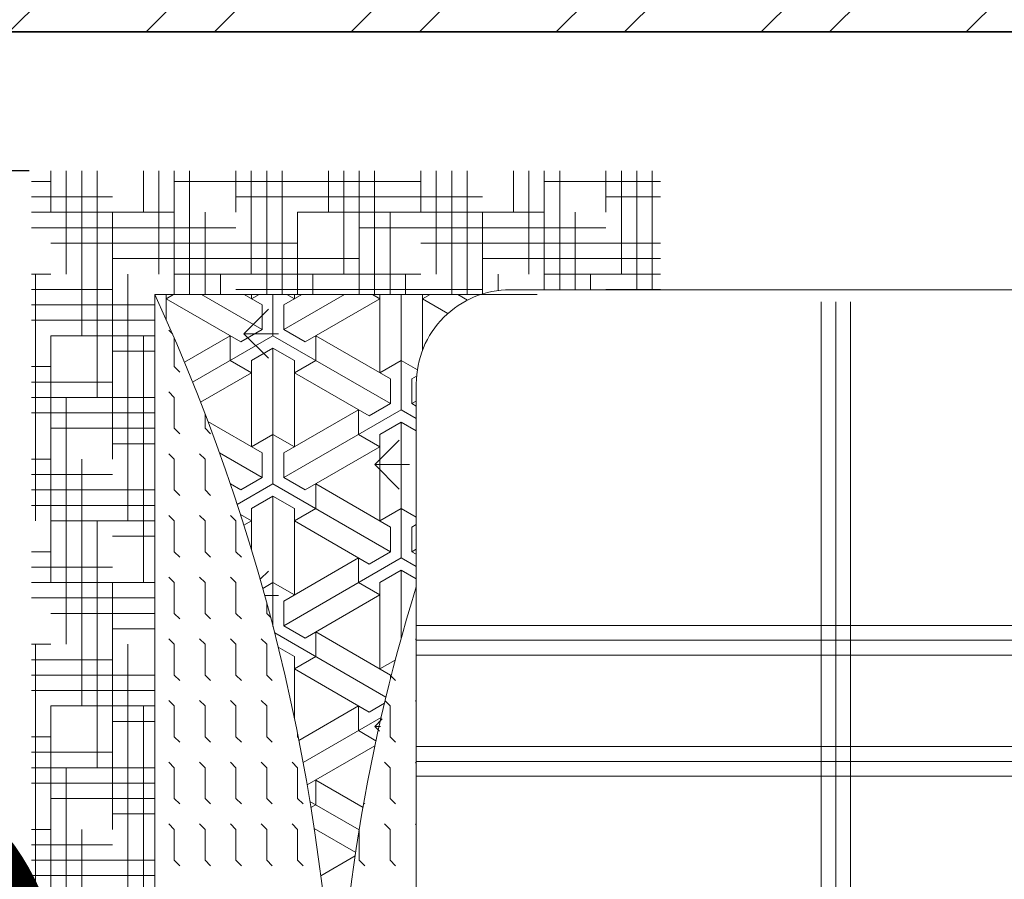
# Model space of a CAD drawing. Units: inches. Extents: x -90 to 536, y -553 to 299.
# Tile 7 of 27: x 96 to 122, y -362 to -339. Entities that reach past the tile are written whole.
import ezdxf

# ---------------------------------------------------------------- set-up
doc = ezdxf.new("R2010")
doc.units = ezdxf.units.IN
for name, color, linetype, lineweight in [('A-ANNO-DIMS', 2, 'Continuous', 18), ('A-WALL-PATT', 252, 'Continuous', 13), ('Furniture', 2, 'Continuous', 18), ('Inner Wall', 5, 'Continuous', 35)]:
    doc.layers.add(name, color=color, linetype=linetype, lineweight=lineweight)
doc.styles.get("Standard").update_dxf_attribs({"font": 'arial.ttf'})
doc.dimstyles.get("Standard").update_dxf_attribs({"dimtxt": 18, "dimasz": 12, "dimexe": 0.18, "dimexo": 0.0625, "dimgap": 0.09, "dimtad": 0, "dimtih": 1, "dimtoh": 1, "dimdec": 0, "dimzin": 0, "dimdsep": 46, "dimlunit": 3, "dimtxsty": 'Standard', "dimcen": 0.09, "dimadec": 0, "dimazin": 0, "dimtfac": 1, "dimtdec": 0, "dimtofl": 0, "dimtmove": 0, "dimatfit": 3, "dimfxl": 1, "dimtolj": 1, "dimtzin": 0, "dimarcsym": 0})

# ---------------------------------------------------------------- blocks, each defined once
blk = doc.blocks.new('A$C62731D1C')
for p, q in [((0.09627, 0.38824, 0.68571), (0.09627, 2.14084, 0.68571)), ((0.46643, 1.44371, 0.68571), (0.46643, 0.31204, 0.68571)), ((0.47843, 1.44371, 0.68571), (0.47843, 0.31204, 0.68571)), ((0.49043, 1.44371, 0.68571), (0.49043, 0.31204, 0.68571)), ((0.36826, 1.4076, 0.68571), (0.36826, 0.31204, 0.68571)), ((0.38026, 1.4076, 0.68571), (0.38026, 0.31204, 0.68571)), ((0.39226, 1.4076, 0.68571), (0.39226, 0.31204, 0.68571)), ((0.10613, 0.66415, 0.68571), (1.46095, 0.66415, 0.68571)), ((0.10613, 0.65215, 0.68571), (1.46095, 0.65215, 0.68571)), ((0.10613, 0.64015, 0.68571), (1.46095, 0.64015, 0.68571)), ((0, 0.50327, 0.68571), (0.09627, 0.50327, 0.68571)), ((0.0085, 0.41577, 0.68571), (0.0085, 0.50998, 0.68571)), ((0.021, 0.46577, 0.68571), (0.021, 0.50998, 0.68571)), ((0.0585, 0.31577, 0.68571), (0.0585, 0.50998, 0.68571)), ((0.071, 0.36577, 0.68571), (0.071, 0.50998, 0.68571)), ((0.0835, 0.41577, 0.68571), (0.0835, 0.50998, 0.68571)), ((0.096, 0.46577, 0.68571), (0.096, 0.50998, 0.68571)), ((0, 0.49077, 0.68571), (0.09627, 0.49077, 0.68571)), ((0, 0.47827, 0.68571), (0.0835, 0.47827, 0.68571)), ((0, 0.46577, 0.68571), (0.0335, 0.46577, 0.68571)), ((0.046, 0.26577, 0.68571), (0.046, 0.46577, 0.68571)), ((0.0835, 0.45327, 0.68571), (0.09627, 0.45327, 0.68571)), ((0.0335, 0.44077, 0.68571), (0.09627, 0.44077, 0.68571)), ((0, 0.42827, 0.68571), (0.09627, 0.42827, 0.68571)), ((0, 0.41577, 0.68571), (0.09627, 0.41577, 0.68571)), ((0.0335, 0.21577, 0.68571), (0.0335, 0.41577, 0.68571)), ((0.1, 0.1, 0.68571), (0.1, 0.40998, 0.68571)), ((0, 0.40327, 0.68571), (0.0835, 0.40327, 0.68571)), ((0, 0.39077, 0.68571), (0.0335, 0.39077, 0.68571)), ((0.0835, 0.37827, 0.68571), (0.09693, 0.37827, 0.68571)), ((0.021, 0.16577, 0.68571), (0.021, 0.36577, 0.68571)), ((0.0335, 0.36577, 0.68571), (0.09966, 0.36577, 0.68571)), ((0.096, 0.16577, 0.68571), (0.096, 0.36577, 0.68571)), ((0, 0.35327, 0.68571), (0.1, 0.35327, 0.68571)), ((0.1, 0.34567, 0.68571), (0.10459, 0.35362, 0.68571)), ((0, 0.34077, 0.68571), (0.1, 0.34077, 0.68571)), ((0.11542, 0.33773, 0.68571), (0.1035, 0.31709, 0.68571)), ((0, 0.32827, 0.68571), (0.0835, 0.32827, 0.68571)), ((0.1, 0.32316, 0.68571), (0.1035, 0.31709, 0.68571)), ((0, 0.31577, 0.68571), (0.0335, 0.31577, 0.68571)), ((0.0085, 0.11577, 0.68571), (0.0085, 0.31577, 0.68571)), ((0.0835, 0.11577, 0.68571), (0.0835, 0.31577, 0.68571)), ((0.1, 0.31709, 0.68571), (0.14518, 0.31709, 0.68571)), ((0.1535, 0.29977, 0.68571), (0.16108, 0.3129, 0.68571)), ((0.1685, 0.30843, 0.68571), (0.16627, 0.31229, 0.68571)), ((1.39167, 0.31204, 0.68571), (0.17247, 0.31204, 0.68571)), ((0.18642, 0.31204, 0.68571), (0.1885, 0.30843, 0.68571)), ((0.1885, 0.30843, 0.68571), (0.19058, 0.31204, 0.68571)), ((0.1935, 0.29977, 0.68571), (0.20058, 0.31204, 0.68571)), ((0.2035, 0.29977, 0.68571), (0.21058, 0.31204, 0.68571)), ((0.2735, 0.29977, 0.68571), (0.28058, 0.31204, 0.68571)), ((0.2885, 0.30843, 0.68571), (0.28642, 0.31204, 0.68571)), ((0.30642, 0.31204, 0.68571), (0.3085, 0.30843, 0.68571)), ((0.3085, 0.30843, 0.68571), (0.31058, 0.31204, 0.68571)), ((0.3135, 0.29977, 0.68571), (0.32058, 0.31204, 0.68571)), ((0.3235, 0.29977, 0.68571), (0.33058, 0.31204, 0.68571)), ((0.37908, 0.31135, 0.68571), (0.37977, 0.31204, 0.68571)), ((0.42908, 0.31135, 0.68571), (0.42977, 0.31204, 0.68571)), ((0.47908, 0.31135, 0.68571), (0.47977, 0.31204, 0.68571)), ((0.52908, 0.31135, 0.68571), (0.52977, 0.31204, 0.68571)), ((0.1885, 0.30843, 0.68571), (0.1685, 0.30843, 0.68571)), ((0.23796, 0.2783, 0.68571), (0.23796, 0.30643, 0.68571)), ((0.3085, 0.30843, 0.68571), (0.2885, 0.30843, 0.68571)), ((0.0835, 0.30327, 0.68571), (0.1, 0.30327, 0.68571)), ((0.1935, 0.29977, 0.68571), (0.1, 0.29977, 0.68571)), ((0.1535, 0.29977, 0.68571), (0.1635, 0.28245, 0.68571)), ((0.1935, 0.29977, 0.68571), (0.2485, 0.20451, 0.68571)), ((0.3135, 0.29977, 0.68571), (0.2035, 0.29977, 0.68571)), ((0.2035, 0.29977, 0.68571), (0.2135, 0.28245, 0.68571)), ((0.23796, 0.2783, 0.68571), (0.21807, 0.29819, 0.68571)), ((0.23796, 0.2783, 0.68571), (0.25785, 0.29819, 0.68571)), ((0.2735, 0.29977, 0.68571), (0.2835, 0.28245, 0.68571)), ((0.3135, 0.29977, 0.68571), (0.3685, 0.20451, 0.68571)), ((0.37861, 0.29977, 0.68571), (0.3235, 0.29977, 0.68571)), ((0.3235, 0.29977, 0.68571), (0.3335, 0.28245, 0.68571)), ((0.0335, 0.29077, 0.68571), (0.1, 0.29077, 0.68571)), ((0.1335, 0.19585, 0.68571), (0.1885, 0.29111, 0.68571)), ((0.1685, 0.29111, 0.68571), (0.1335, 0.23049, 0.68571)), ((0.1885, 0.29111, 0.68571), (0.1685, 0.29111, 0.68571)), ((0.1885, 0.29111, 0.68571), (0.1985, 0.27379, 0.68571)), ((0.2535, 0.19585, 0.68571), (0.3085, 0.29111, 0.68571)), ((0.2885, 0.29111, 0.68571), (0.2535, 0.23049, 0.68571)), ((0.3085, 0.29111, 0.68571), (0.2885, 0.29111, 0.68571)), ((0.3085, 0.29111, 0.68571), (0.3185, 0.27379, 0.68571)), ((0.4085, 0.29111, 0.68571), (0.3735, 0.23049, 0.68571)), ((0.37428, 0.19721, 0.68571), (0.42636, 0.2874, 0.68571)), ((0.39626, 0.295, 0.68571), (0.4035, 0.28245, 0.68571)), ((0.4113, 0.29111, 0.68571), (0.4085, 0.29111, 0.68571)), ((0.40934, 0.29161, 0.68571), (0.41292, 0.29519, 0.68571)), ((0.4294, 0.28667, 0.68571), (0.4335, 0.29077, 0.68571)), ((0.4335, 0.29077, 0.68571), (0.4585, 0.29077, 0.68571)), ((0.4585, 0.29077, 0.68571), (0.46292, 0.29519, 0.68571)), ((0.47908, 0.28635, 0.68571), (0.4835, 0.29077, 0.68571)), ((0.4835, 0.29077, 0.68571), (0.5085, 0.29077, 0.68571)), ((0.5085, 0.29077, 0.68571), (0.51292, 0.29519, 0.68571)), ((0.52908, 0.28635, 0.68571), (0.5335, 0.29077, 0.68571)), ((0.5335, 0.29077, 0.68571), (0.5585, 0.29077, 0.68571)), ((0.5585, 0.29077, 0.68571), (0.56292, 0.29519, 0.68571)), ((0.1, 0.27639, 0.68571), (0.1035, 0.28245, 0.68571)), ((0.1, 0.28245, 0.68571), (0.1635, 0.28245, 0.68571)), ((0.1385, 0.22183, 0.68571), (0.1035, 0.28245, 0.68571)), ((0.2135, 0.26513, 0.68571), (0.2235, 0.28245, 0.68571)), ((0.2135, 0.28245, 0.68571), (0.2835, 0.28245, 0.68571)), ((0.2585, 0.22183, 0.68571), (0.2235, 0.28245, 0.68571)), ((0.3335, 0.26513, 0.68571), (0.3435, 0.28245, 0.68571)), ((0.3335, 0.28245, 0.68571), (0.4035, 0.28245, 0.68571)), ((0.3785, 0.22183, 0.68571), (0.3435, 0.28245, 0.68571)), ((0.43133, 0.28621, 0.68571), (0.4385, 0.27379, 0.68571)), ((0.44289, 0.28352, 0.68571), (0.47937, 0.22033, 0.68571)), ((0.45009, 0.2783, 0.68571), (0.44401, 0.28439, 0.68571)), ((0.45009, 0.2783, 0.68571), (0.45009, 0.28301, 0.68571)), ((0.45009, 0.2783, 0.68571), (0.45394, 0.28215, 0.68571)), ((0, 0.27827, 0.68571), (0.1, 0.27827, 0.68571)), ((0.1985, 0.27379, 0.68571), (0.1635, 0.21317, 0.68571)), ((0.3185, 0.27379, 0.68571), (0.2835, 0.21317, 0.68571)), ((0.4385, 0.27379, 0.68571), (0.4035, 0.21317, 0.68571)), ((0.4535, 0.26513, 0.68571), (0.46171, 0.27934, 0.68571)), ((0.49749, 0.22358, 0.68571), (0.4658, 0.27847, 0.68571)), ((0, 0.26577, 0.68571), (0.1, 0.26577, 0.68571)), ((0.071, 0.06577, 0.68571), (0.071, 0.26577, 0.68571)), ((0.2135, 0.26513, 0.68571), (0.1935, 0.26513, 0.68571)), ((0.2285, 0.20451, 0.68571), (0.1935, 0.26513, 0.68571)), ((0.3335, 0.26513, 0.68571), (0.3135, 0.26513, 0.68571)), ((0.3485, 0.20451, 0.68571), (0.3135, 0.26513, 0.68571)), ((0.4535, 0.26513, 0.68571), (0.4335, 0.26513, 0.68571)), ((0.46136, 0.21689, 0.68571), (0.4335, 0.26513, 0.68571)), ((0.51564, 0.26884, 0.68571), (0.4935, 0.23049, 0.68571)), ((0.51081, 0.22583, 0.68571), (0.53387, 0.26577, 0.68571)), ((0.51218, 0.26945, 0.68571), (0.51292, 0.27019, 0.68571)), ((0.53385, 0.26577, 0.68571), (0.5585, 0.26577, 0.68571)), ((0.5585, 0.26577, 0.68571), (0.56292, 0.27019, 0.68571)), ((0.55222, 0.26292, 0.68571), (0.53281, 0.2293, 0.68571)), ((0.57113, 0.2346, 0.68571), (0.55502, 0.2625, 0.68571)), ((0, 0.25327, 0.68571), (0.0835, 0.25327, 0.68571)), ((0.1, 0.25388, 0.68571), (0.1285, 0.20451, 0.68571)), ((0, 0.24077, 0.68571), (0.0335, 0.24077, 0.68571)), ((0.0835, 0.22827, 0.68571), (0.1, 0.22827, 0.68571)), ((0.1535, 0.23049, 0.68571), (0.1335, 0.23049, 0.68571)), ((0.1535, 0.23049, 0.68571), (0.1635, 0.21317, 0.68571)), ((0.2735, 0.23049, 0.68571), (0.2535, 0.23049, 0.68571)), ((0.2735, 0.23049, 0.68571), (0.2835, 0.21317, 0.68571)), ((0.3935, 0.23049, 0.68571), (0.3735, 0.23049, 0.68571)), ((0.3935, 0.23049, 0.68571), (0.4035, 0.21317, 0.68571)), ((0.5135, 0.23049, 0.68571), (0.4935, 0.23049, 0.68571)), ((0.5135, 0.23049, 0.68571), (0.51573, 0.22663, 0.68571)), ((0.0335, 0.21577, 0.68571), (0.1, 0.21577, 0.68571)), ((0.0585, 0.01577, 0.68571), (0.0585, 0.21577, 0.68571)), ((0.1085, 0.20451, 0.68571), (0.1, 0.21924, 0.68571)), ((0.1285, 0.20451, 0.68571), (0.1385, 0.22183, 0.68571)), ((0.2485, 0.20451, 0.68571), (0.2585, 0.22183, 0.68571)), ((0.3685, 0.20451, 0.68571), (0.3785, 0.22183, 0.68571)), ((0.45574, 0.21577, 0.68571), (0.4585, 0.21577, 0.68571)), ((0.4585, 0.21577, 0.68571), (0.45919, 0.21646, 0.68571)), ((0.47908, 0.21135, 0.68571), (0.4835, 0.21577, 0.68571)), ((0.4835, 0.21577, 0.68571), (0.5085, 0.21577, 0.68571)), ((0.5085, 0.21577, 0.68571), (0.51292, 0.22019, 0.68571)), ((0.52908, 0.21135, 0.68571), (0.5335, 0.21577, 0.68571)), ((0.5335, 0.21577, 0.68571), (0.5585, 0.21577, 0.68571)), ((0.5585, 0.21577, 0.68571), (0.56292, 0.22019, 0.68571)), ((0.1, 0.20711, 0.68571), (0.1035, 0.21317, 0.68571)), ((0.1, 0.21317, 0.68571), (0.1035, 0.21317, 0.68571)), ((0.1435, 0.19585, 0.68571), (0.1535, 0.21317, 0.68571)), ((0.1535, 0.21317, 0.68571), (0.2235, 0.21317, 0.68571)), ((0.2135, 0.19585, 0.68571), (0.2235, 0.21317, 0.68571)), ((0.2635, 0.19585, 0.68571), (0.2735, 0.21317, 0.68571)), ((0.2735, 0.21317, 0.68571), (0.3435, 0.21317, 0.68571)), ((0.3335, 0.19585, 0.68571), (0.3435, 0.21317, 0.68571)), ((0.38598, 0.20015, 0.68571), (0.3935, 0.21317, 0.68571)), ((0.3935, 0.21317, 0.68571), (0.44307, 0.21317, 0.68571)), ((0, 0.20327, 0.68571), (0.1, 0.20327, 0.68571)), ((0.1285, 0.20451, 0.68571), (0.1085, 0.20451, 0.68571)), ((0.13189, 0.17223, 0.68571), (0.13189, 0.20036, 0.68571)), ((0.2485, 0.20451, 0.68571), (0.2285, 0.20451, 0.68571)), ((0.34403, 0.18916, 0.68571), (0.34403, 0.20036, 0.68571)), ((0.3685, 0.20451, 0.68571), (0.3485, 0.20451, 0.68571)), ((0.1335, 0.19585, 0.68571), (0.1, 0.19585, 0.68571)), ((0.13189, 0.17223, 0.68571), (0.11201, 0.19212, 0.68571)), ((0.13189, 0.17223, 0.68571), (0.15178, 0.19212, 0.68571)), ((0.1335, 0.19585, 0.68571), (0.17113, 0.13067, 0.68571)), ((0.2535, 0.19585, 0.68571), (0.1435, 0.19585, 0.68571)), ((0.1435, 0.19585, 0.68571), (0.1535, 0.17853, 0.68571)), ((0.2135, 0.19585, 0.68571), (0.2235, 0.17853, 0.68571)), ((0.2535, 0.19585, 0.68571), (0.27024, 0.16687, 0.68571)), ((0.36902, 0.19585, 0.68571), (0.2635, 0.19585, 0.68571)), ((0.2635, 0.19585, 0.68571), (0.2735, 0.17853, 0.68571)), ((0.33081, 0.18545, 0.68571), (0.32414, 0.19212, 0.68571)), ((0.3335, 0.19585, 0.68571), (0.33829, 0.18757, 0.68571)), ((0.3585, 0.19077, 0.68571), (0.36166, 0.19393, 0.68571)), ((0.4085, 0.19077, 0.68571), (0.41292, 0.19519, 0.68571)), ((0.4585, 0.19077, 0.68571), (0.46292, 0.19519, 0.68571)), ((0.5085, 0.19077, 0.68571), (0.51292, 0.19519, 0.68571)), ((0.5585, 0.19077, 0.68571), (0.56292, 0.19519, 0.68571)), ((0, 0.19077, 0.68571), (0.1, 0.19077, 0.68571)), ((0.1, 0.13782, 0.68571), (0.1285, 0.18719, 0.68571)), ((0.1085, 0.18719, 0.68571), (0.1, 0.17247, 0.68571)), ((0.1, 0.1846, 0.68571), (0.1035, 0.17853, 0.68571)), ((0.1285, 0.18719, 0.68571), (0.1085, 0.18719, 0.68571)), ((0.1285, 0.18719, 0.68571), (0.1385, 0.16987, 0.68571)), ((0.2285, 0.18719, 0.68571), (0.20307, 0.14314, 0.68571)), ((0.22848, 0.15251, 0.68571), (0.2485, 0.18719, 0.68571)), ((0.2485, 0.18719, 0.68571), (0.2285, 0.18719, 0.68571)), ((0.2485, 0.18719, 0.68571), (0.2585, 0.16987, 0.68571)), ((0.34988, 0.19077, 0.68571), (0.3585, 0.19077, 0.68571)), ((0.37908, 0.18635, 0.68571), (0.3835, 0.19077, 0.68571)), ((0.3835, 0.19077, 0.68571), (0.4085, 0.19077, 0.68571)), ((0.42908, 0.18635, 0.68571), (0.4335, 0.19077, 0.68571)), ((0.4335, 0.19077, 0.68571), (0.4585, 0.19077, 0.68571)), ((0.47908, 0.18635, 0.68571), (0.4835, 0.19077, 0.68571)), ((0.4835, 0.19077, 0.68571), (0.5085, 0.19077, 0.68571)), ((0.52908, 0.18635, 0.68571), (0.5335, 0.19077, 0.68571)), ((0.5335, 0.19077, 0.68571), (0.5585, 0.19077, 0.68571)), ((0, 0.17827, 0.68571), (0.0835, 0.17827, 0.68571)), ((0.1, 0.17853, 0.68571), (0.1035, 0.17853, 0.68571)), ((0.1535, 0.16121, 0.68571), (0.1635, 0.17853, 0.68571)), ((0.1535, 0.17853, 0.68571), (0.2235, 0.17853, 0.68571)), ((0.18741, 0.13712, 0.68571), (0.1635, 0.17853, 0.68571)), ((0.2735, 0.17853, 0.68571), (0.30724, 0.17853, 0.68571)), ((0.27828, 0.16948, 0.68571), (0.2835, 0.17853, 0.68571)), ((0.2871, 0.1723, 0.68571), (0.2835, 0.17853, 0.68571)), ((0.1385, 0.16987, 0.68571), (0.1035, 0.10925, 0.68571)), ((0.2585, 0.16987, 0.68571), (0.25354, 0.16128, 0.68571)), ((0.3085, 0.16577, 0.68571), (0.31292, 0.17019, 0.68571)), ((0.3585, 0.16577, 0.68571), (0.36292, 0.17019, 0.68571)), ((0.4085, 0.16577, 0.68571), (0.41292, 0.17019, 0.68571)), ((0.4585, 0.16577, 0.68571), (0.46292, 0.17019, 0.68571)), ((0.5085, 0.16577, 0.68571), (0.51292, 0.17019, 0.68571)), ((0.5585, 0.16577, 0.68571), (0.56292, 0.17019, 0.68571)), ((0, 0.16577, 0.68571), (0.0335, 0.16577, 0.68571)), ((0.046, 0, 0.68571), (0.046, 0.16577, 0.68571)), ((0.1535, 0.16121, 0.68571), (0.1335, 0.16121, 0.68571)), ((0.15496, 0.12405, 0.68571), (0.1335, 0.16121, 0.68571)), ((0.27908, 0.16135, 0.68571), (0.2835, 0.16577, 0.68571)), ((0.2835, 0.16577, 0.68571), (0.3085, 0.16577, 0.68571)), ((0.32908, 0.16135, 0.68571), (0.3335, 0.16577, 0.68571)), ((0.3335, 0.16577, 0.68571), (0.3585, 0.16577, 0.68571)), ((0.37908, 0.16135, 0.68571), (0.3835, 0.16577, 0.68571)), ((0.3835, 0.16577, 0.68571), (0.4085, 0.16577, 0.68571)), ((0.42908, 0.16135, 0.68571), (0.4335, 0.16577, 0.68571)), ((0.4335, 0.16577, 0.68571), (0.4585, 0.16577, 0.68571)), ((0.47908, 0.16135, 0.68571), (0.4835, 0.16577, 0.68571)), ((0.4835, 0.16577, 0.68571), (0.5085, 0.16577, 0.68571)), ((0.52908, 0.16135, 0.68571), (0.5335, 0.16577, 0.68571)), ((0.5335, 0.16577, 0.68571), (0.5585, 0.16577, 0.68571)), ((0.0835, 0.15327, 0.68571), (0.1, 0.15327, 0.68571)), ((0.2085, 0.14077, 0.68571), (0.21292, 0.14519, 0.68571)), ((0.2585, 0.14077, 0.68571), (0.26292, 0.14519, 0.68571)), ((0.3085, 0.14077, 0.68571), (0.31292, 0.14519, 0.68571)), ((0.3585, 0.14077, 0.68571), (0.36292, 0.14519, 0.68571)), ((0.4085, 0.14077, 0.68571), (0.41292, 0.14519, 0.68571)), ((0.4585, 0.14077, 0.68571), (0.46292, 0.14519, 0.68571)), ((0.5085, 0.14077, 0.68571), (0.51292, 0.14519, 0.68571)), ((0.5585, 0.14077, 0.68571), (0.56292, 0.14519, 0.68571)), ((0.0335, 0.14077, 0.68571), (0.1, 0.14077, 0.68571)), ((0.19684, 0.14077, 0.68571), (0.2085, 0.14077, 0.68571)), ((0.22908, 0.13635, 0.68571), (0.2335, 0.14077, 0.68571)), ((0.2335, 0.14077, 0.68571), (0.2585, 0.14077, 0.68571)), ((0.27908, 0.13635, 0.68571), (0.2835, 0.14077, 0.68571)), ((0.2835, 0.14077, 0.68571), (0.3085, 0.14077, 0.68571)), ((0.32908, 0.13635, 0.68571), (0.3335, 0.14077, 0.68571)), ((0.3335, 0.14077, 0.68571), (0.3585, 0.14077, 0.68571)), ((0.37908, 0.13635, 0.68571), (0.3835, 0.14077, 0.68571)), ((0.3835, 0.14077, 0.68571), (0.4085, 0.14077, 0.68571)), ((0.42908, 0.13635, 0.68571), (0.4335, 0.14077, 0.68571)), ((0.4335, 0.14077, 0.68571), (0.4585, 0.14077, 0.68571)), ((0.47908, 0.13635, 0.68571), (0.4835, 0.14077, 0.68571)), ((0.4835, 0.14077, 0.68571), (0.5085, 0.14077, 0.68571)), ((0.52908, 0.13635, 0.68571), (0.5335, 0.14077, 0.68571)), ((0.5335, 0.14077, 0.68571), (0.5585, 0.14077, 0.68571)), ((0, 0.12827, 0.68571), (0.1, 0.12827, 0.68571)), ((0.1585, 0.11577, 0.68571), (0.16292, 0.12019, 0.68571)), ((0.2085, 0.11577, 0.68571), (0.21292, 0.12019, 0.68571)), ((0.2585, 0.11577, 0.68571), (0.26292, 0.12019, 0.68571)), ((0.3085, 0.11577, 0.68571), (0.31292, 0.12019, 0.68571)), ((0.3585, 0.11577, 0.68571), (0.36292, 0.12019, 0.68571)), ((0.4085, 0.11577, 0.68571), (0.41292, 0.12019, 0.68571)), ((0.4585, 0.11577, 0.68571), (0.46292, 0.12019, 0.68571)), ((0.5085, 0.11577, 0.68571), (0.51292, 0.12019, 0.68571)), ((0.5585, 0.11577, 0.68571), (0.56292, 0.12019, 0.68571)), ((0, 0.11577, 0.68571), (0.1, 0.11577, 0.68571)), ((0.0335, 0, 0.68571), (0.0335, 0.11577, 0.68571)), ((0.1, 0.11531, 0.68571), (0.1035, 0.10925, 0.68571)), ((0.12908, 0.11135, 0.68571), (0.13206, 0.11432, 0.68571)), ((0.1354, 0.11577, 0.68571), (0.1585, 0.11577, 0.68571)), ((0.17908, 0.11135, 0.68571), (0.1835, 0.11577, 0.68571)), ((0.1835, 0.11577, 0.68571), (0.2085, 0.11577, 0.68571)), ((0.22908, 0.11135, 0.68571), (0.2335, 0.11577, 0.68571)), ((0.2335, 0.11577, 0.68571), (0.2585, 0.11577, 0.68571)), ((0.27908, 0.11135, 0.68571), (0.2835, 0.11577, 0.68571)), ((0.2835, 0.11577, 0.68571), (0.3085, 0.11577, 0.68571)), ((0.32908, 0.11135, 0.68571), (0.3335, 0.11577, 0.68571)), ((0.3335, 0.11577, 0.68571), (0.3585, 0.11577, 0.68571)), ((0.37908, 0.11135, 0.68571), (0.3835, 0.11577, 0.68571)), ((0.3835, 0.11577, 0.68571), (0.4085, 0.11577, 0.68571)), ((0.42908, 0.11135, 0.68571), (0.4335, 0.11577, 0.68571)), ((0.4335, 0.11577, 0.68571), (0.4585, 0.11577, 0.68571)), ((0.47908, 0.11135, 0.68571), (0.4835, 0.11577, 0.68571)), ((0.4835, 0.11577, 0.68571), (0.5085, 0.11577, 0.68571)), ((0.52908, 0.11135, 0.68571), (0.5335, 0.11577, 0.68571)), ((0.5335, 0.11577, 0.68571), (0.5585, 0.11577, 0.68571)), ((0.1, 0.10925, 0.68571), (0.12048, 0.10925, 0.68571)), ((0, 0.10327, 0.68571), (0.0835, 0.10327, 0.68571)), ((1.44488, 0.1, 0.68571), (0.1, 0.1, 0.68571)), ((0.1085, 0, 0.68571), (0.1085, 0.1, 0.68571)), ((0.121, 0, 0.68571), (0.121, 0.1, 0.68571)), ((0.1335, 0.01577, 0.68571), (0.1335, 0.1, 0.68571)), ((0.146, 0.06577, 0.68571), (0.146, 0.1, 0.68571)), ((0.1835, 0, 0.68571), (0.1835, 0.1, 0.68571)), ((0.196, 0, 0.68571), (0.196, 0.1, 0.68571)), ((0.2085, 0.01577, 0.68571), (0.2085, 0.1, 0.68571)), ((0.221, 0.06577, 0.68571), (0.221, 0.1, 0.68571)), ((0.2585, 0, 0.68571), (0.2585, 0.1, 0.68571)), ((0.271, 0, 0.68571), (0.271, 0.1, 0.68571)), ((0.2835, 0.01577, 0.68571), (0.2835, 0.1, 0.68571)), ((0.296, 0.06577, 0.68571), (0.296, 0.1, 0.68571)), ((0.3335, 0, 0.68571), (0.3335, 0.1, 0.68571)), ((0.346, 0, 0.68571), (0.346, 0.1, 0.68571)), ((0.3585, 0.01577, 0.68571), (0.3585, 0.1, 0.68571)), ((0.371, 0.06577, 0.68571), (0.371, 0.1, 0.68571)), ((0.4085, 0, 0.68571), (0.4085, 0.1, 0.68571)), ((0.421, 0, 0.68571), (0.421, 0.1, 0.68571)), ((0.4335, 0.01577, 0.68571), (0.4335, 0.1, 0.68571)), ((0.446, 0.06577, 0.68571), (0.446, 0.1, 0.68571)), ((0.4835, 0, 0.68571), (0.4835, 0.1, 0.68571)), ((0.496, 0, 0.68571), (0.496, 0.1, 0.68571)), ((0.5085, 0.01577, 0.68571), (0.5085, 0.1, 0.68571)), ((0.521, 0.06577, 0.68571), (0.521, 0.1, 0.68571)), ((0.5585, 0, 0.68571), (0.5585, 0.1, 0.68571)), ((0.571, 0, 0.68571), (0.571, 0.1, 0.68571)), ((0, 0.09077, 0.68571), (0.0335, 0.09077, 0.68571)), ((0.1335, 0.09077, 0.68571), (0.3335, 0.09077, 0.68571)), ((0.4335, 0.09077, 0.68571), (0.6335, 0.09077, 0.68571)), ((0.0835, 0.07827, 0.68571), (0.2835, 0.07827, 0.68571)), ((0.3835, 0.07827, 0.68571), (0.5835, 0.07827, 0.68571)), ((0.021, 0, 0.68571), (0.021, 0.06577, 0.68571)), ((0.0335, 0.06577, 0.68571), (0.2335, 0.06577, 0.68571)), ((0.096, 0, 0.68571), (0.096, 0.06577, 0.68571)), ((0.171, 0, 0.68571), (0.171, 0.06577, 0.68571)), ((0.246, 0, 0.68571), (0.246, 0.06577, 0.68571)), ((0.321, 0, 0.68571), (0.321, 0.06577, 0.68571)), ((0.3335, 0.06577, 0.68571), (0.5335, 0.06577, 0.68571)), ((0.396, 0, 0.68571), (0.396, 0.06577, 0.68571)), ((0.471, 0, 0.68571), (0.471, 0.06577, 0.68571)), ((0.546, 0, 0.68571), (0.546, 0.06577, 0.68571)), ((0, 0.05327, 0.68571), (0.1835, 0.05327, 0.68571)), ((0.2835, 0.05327, 0.68571), (0.4835, 0.05327, 0.68571)), ((0, 0.04077, 0.68571), (0.1335, 0.04077, 0.68571)), ((0.2335, 0.04077, 0.68571), (0.4335, 0.04077, 0.68571)), ((0.5335, 0.04077, 0.68571), (0.7335, 0.04077, 0.68571)), ((0, 0.02827, 0.68571), (0.0835, 0.02827, 0.68571)), ((0.1835, 0.02827, 0.68571), (0.3835, 0.02827, 0.68571)), ((0.4835, 0.02827, 0.68571), (0.6835, 0.02827, 0.68571)), ((0, 0.01577, 0.68571), (0.0335, 0.01577, 0.68571)), ((0.0085, 0, 0.68571), (0.0085, 0.01577, 0.68571)), ((0.0835, 0, 0.68571), (0.0835, 0.01577, 0.68571)), ((0.1335, 0.01577, 0.68571), (0.3335, 0.01577, 0.68571)), ((0.1585, 0, 0.68571), (0.1585, 0.01577, 0.68571)), ((0.2335, 0, 0.68571), (0.2335, 0.01577, 0.68571)), ((0.3085, 0, 0.68571), (0.3085, 0.01577, 0.68571)), ((0.3835, 0, 0.68571), (0.3835, 0.01577, 0.68571)), ((0.4335, 0.01577, 0.68571), (0.6335, 0.01577, 0.68571)), ((0.4585, 0, 0.68571), (0.4585, 0.01577, 0.68571)), ((0.5335, 0, 0.68571), (0.5335, 0.01577, 0.68571)), ((0.0835, 0.00327, 0.68571), (0.2835, 0.00327, 0.68571)), ((0.3835, 0.00327, 0.68571), (0.5835, 0.00327, 0.68571))]:
    blk.add_line(p, q)
for centre, radius, start, end in [((0.17247, 0.38824, 0.68571), 0.0762, 180, 270), ((0.76456, 1.69033, 0.68571), 1.44313, 252.76056, 287.23944), ((0.77244, -1.36185, 0.68571), 1.6091, 65.29791, 114.70209)]:
    blk.add_arc(centre, radius, start, end)
blk = doc.blocks.new('A$C0E6D7E3D')
blk.add_blockref('A$C62731D1C', (0, 0))
blk = doc.blocks.new('*D28')
at = {"layer": 'A-ANNO-DIMS', "color": 0, "lineweight": -2, "transparency": 16777216}
for p, q in [((92.257, -392.554), (92.257, -380.554)), ((92.257, -380.554), (104.257, -380.554)), ((86.694, -392.554), (92.437, -392.554)), ((92.257, -416.554), (92.257, -404.554)), ((86.694, -428.554), (92.437, -428.554))]:
    blk.add_line(p, q, dxfattribs=at)
at = {"layer": 'A-ANNO-DIMS', "color": 0, "transparency": 16777216}
for points in [[(90.257, -404.554), (94.257, -404.554), (92.257, -392.554)], [(90.257, -416.554), (94.257, -416.554), (92.257, -428.554)]]:
    blk.add_solid(points, dxfattribs=at)
at = {"layer": 'Defpoints', "color": 0, "transparency": 16777216}
for p in [(86.632, -392.554), (92.257, -392.554), (86.632, -428.554)]:
    blk.add_point(p, dxfattribs=at)
at = {"layer": 'A-ANNO-DIMS', "color": 0, "transparency": 16777216, "insert": (148.15, -380.554), "char_height": 18, "attachment_point": 5}
blk.add_mtext('\\A1;36 TYP.', dxfattribs=at)
blk = doc.blocks.new('*D46')
at = {"layer": 'A-ANNO-DIMS', "color": 0, "lineweight": -2, "transparency": 16777216}
for p, q in [((92.796, -304.194), (92.796, -292.194)), ((96.856, -316.194), (92.616, -316.194)), ((96.856, -332.226), (92.616, -332.226)), ((92.796, -344.226), (92.796, -356.226)), ((92.796, -356.226), (80.796, -356.226))]:
    blk.add_line(p, q, dxfattribs=at)
at = {"layer": 'A-ANNO-DIMS', "color": 0, "transparency": 16777216}
for points in [[(90.796, -304.194), (94.796, -304.194), (92.796, -316.194)], [(90.796, -344.226), (94.796, -344.226), (92.796, -332.226)]]:
    blk.add_solid(points, dxfattribs=at)
at = {"layer": 'Defpoints', "color": 0, "transparency": 16777216}
for p in [(96.919, -316.194), (92.796, -332.226), (96.919, -332.226)]:
    blk.add_point(p, dxfattribs=at)
at = {"layer": 'A-ANNO-DIMS', "color": 0, "transparency": 16777216, "insert": (68.667, -356.226), "char_height": 18, "attachment_point": 5}
blk.add_mtext('\\A1;16', dxfattribs=at)
blk = doc.blocks.new('*D52')
at = {"layer": 'A-ANNO-DIMS', "color": 0, "lineweight": -2, "transparency": 16777216}
for p, q in [((96.743, -343.206), (85.477, -343.206)), ((85.657, -355.206), (85.657, -358.961)), ((85.657, -381.277), (85.657, -377.522)), ((96.743, -393.277), (85.477, -393.277))]:
    blk.add_line(p, q, dxfattribs=at)
at = {"layer": 'A-ANNO-DIMS', "color": 0, "transparency": 16777216}
for points in [[(83.657, -355.206), (87.657, -355.206), (85.657, -343.206)], [(83.657, -381.277), (87.657, -381.277), (85.657, -393.277)]]:
    blk.add_solid(points, dxfattribs=at)
at = {"layer": 'Defpoints', "color": 0, "transparency": 16777216}
for p in [(96.806, -343.206), (85.657, -393.277), (96.806, -393.277)]:
    blk.add_point(p, dxfattribs=at)
at = {"layer": 'A-ANNO-DIMS', "color": 0, "transparency": 16777216, "insert": (85.657, -368.242), "char_height": 18, "attachment_point": 5}
blk.add_mtext('\\A1;50', dxfattribs=at)
blk = doc.blocks.new('*D54')
at = {"layer": 'A-ANNO-DIMS', "color": 0, "lineweight": -2, "transparency": 16777216}
for p, q in [((113.069, 249.446), (-2.848, 249.446)), ((-2.668, 237.446), (-2.668, -117.767)), ((-2.668, -491.554), (-2.668, -136.34)), ((38.069, -503.554), (-2.848, -503.554))]:
    blk.add_line(p, q, dxfattribs=at)
at = {"layer": 'A-ANNO-DIMS', "color": 0, "transparency": 16777216}
for points in [[(-4.668, 237.446), (-0.668, 237.446), (-2.668, 249.446)], [(-4.668, -491.554), (-0.668, -491.554), (-2.668, -503.554)]]:
    blk.add_solid(points, dxfattribs=at)
at = {"layer": 'Defpoints', "color": 0, "transparency": 16777216}
for p in [(-2.668, 249.446), (113.132, 249.446), (38.132, -503.554)]:
    blk.add_point(p, dxfattribs=at)
at = {"layer": 'A-ANNO-DIMS', "color": 0, "transparency": 16777216, "insert": (-2.668, -127.054), "char_height": 18, "attachment_point": 5}
blk.add_mtext('\\A1;753', dxfattribs=at)

msp = doc.modelspace()

# ---------------------------------------------------------------- hatches: boundary and pattern name
at = {"layer": 'A-WALL-PATT'}
h = msp.add_hatch(dxfattribs=at)
h.set_pattern_fill('ANSI32', color=256, scale=0.4)
h.set_pattern_definition([(45, (-88.8105, -603.6155), (-2.694077, 2.694077), []), (45, (-87.0145, -603.6155), (-2.694077, 2.694077), [])])
h.paths.add_polyline_path([(285.1317, 246.4462), (131.1317, 246.4462), (131.1317, 237.4462), (285.1317, 237.4462)])
h.paths.add_polyline_path([(122.1317, 237.4462), (113.1317, 237.4462), (113.1317, 152.4462), (122.1317, 152.4462), (122.1317, 166.4704)])
h.paths.add_polyline_path([(303.1317, 237.4462), (294.1317, 237.4462), (294.1317, 152.4462), (303.1317, 152.4462)])
h.paths.add_polyline_path([(47.1317, 91.9277), (38.1317, 91.9277), (38.1317, -6.5538), (77.1317, -6.5538), (77.1317, 2.4462), (70.5655, 2.4462), (47.1317, 2.4462)])
h.paths.add_polyline_path([(83.052, -61.5538), (47.1317, -61.5538), (47.1317, -24.5538), (38.1317, -24.5538), (38.1317, -70.5538), (74.052, -70.5538), (74.052, -223.5538), (38.1317, -223.5538), (38.1317, -503.5538), (92.1317, -503.5538), (92.1317, -437.5538), (191.1317, -437.5538), (191.1317, -428.5538), (83.1317, -428.5538), (83.1317, -494.5538), (47.1317, -494.5538), (47.1317, -232.5538), (83.052, -232.5538), (83.052, -70.5538)])
h.paths.add_polyline_path([(407.1317, -63.5538), (381.1317, -63.5538), (381.1317, 91.9277), (372.1317, 91.9277), (372.1317, 32.8805), (372.1317, -63.5538), (306.5745, -63.5538), (237.1317, -63.5538), (237.1317, -38.5538), (233.1317, -38.5538), (233.1317, -71.5538), (398.1317, -71.5538), (398.1317, -152.5538), (233.1317, -152.5538), (233.1317, -161.5538), (398.1317, -161.5538), (398.1317, -368.5538), (233.1317, -368.5538), (233.1317, -377.5538), (407.1317, -377.5538), (407.1317, -161.5538)])
h.paths.add_polyline_path([(261.1317, -422.5538), (252.1317, -422.5538), (252.1317, -428.5538), (233.1317, -428.5538), (233.1317, -437.5538), (261.1317, -437.5538)])
h.paths.add_polyline_path([(191.1317, -368.5538), (180.1317, -368.5538), (180.1317, -335.5538), (131.5919, -335.5538), (131.5919, -344.5538), (171.1317, -344.5538), (171.1317, -392.5538), (180.1317, -392.5538), (180.1317, -377.5538), (191.1317, -377.5538)], flags=17)
h.paths.add_polyline_path([(180.1317, -223.5538), (152.1317, -223.5538), (152.1317, -227.5538), (176.1317, -227.5538), (176.1317, -335.5538), (180.1317, -335.5538)], flags=17)
h.paths.add_polyline_path([(131.5919, -335.5538), (83.1317, -335.5538), (83.1317, -339.5538), (83.1317, -392.5538), (87.1317, -392.5538), (87.1317, -339.5538), (131.5919, -339.5538)], flags=17)
h.paths.add_polyline_path([(197.1317, 2.4462), (77.1317, 2.4462), (77.1317, -1.5538), (113.1317, -1.5538), (113.1317, -71.5538), (181.1317, -71.5538), (181.1317, -67.5538), (117.1317, -67.5538), (117.1317, -1.5538), (177.1317, -1.5538), (177.1317, -37.5538), (181.1317, -37.5538), (181.1317, -1.5538), (197.1317, -1.5538)])
h.paths.add_polyline_path([(173.1317, 138.4462), (122.1317, 138.4462), (122.1317, 134.4462), (173.1317, 134.4462)])
h.paths.add_polyline_path([(213.1317, 237.4462), (209.1317, 237.4462), (209.1317, 134.4462), (233.1317, 134.4462), (233.1317, 68.8889), (233.1317, -2.5538), (237.1317, -2.5538), (237.1317, 134.4462), (258.1317, 134.4462), (258.1317, 138.4462), (213.1317, 138.4462)])

# ---------------------------------------------------------------- linework, layer by layer
at = {"layer": 'Inner Wall'}
msp.add_line((87.1317, -339.5538), (131.5919, -339.5538), dxfattribs=at)

# ---------------------------------------------------------------- block references
at = {"layer": 'Furniture', "xscale": 32.41097235378273, "yscale": 32.41097235378273, "zscale": 32.41097235378273, "rotation": 270}
msp.add_blockref('A$C0E6D7E3D', (96.8056, -343.2061, -22.2246), dxfattribs=at)

# ---------------------------------------------------------------- dimensions: what is measured, and where the dimension line sits
at = {"layer": 'A-ANNO-DIMS'}
for base, p1, p2, angle, picture, middle in [((-2.6677, 249.4462), (38.1317, -503.5538), (113.1317, 249.4462), 90, '*D54', (-2.6677, -127.0538)), ((92.7963, -332.2258), (96.9187, -316.194), (96.9187, -332.2258), 270, '*D46', (68.6674, -356.2258)), ((85.6567, -393.2773), (96.8056, -343.2061), (96.8056, -393.2773), 270, '*D52', (85.6567, -368.2417))]:
    dim = msp.add_linear_dim(base=base, p1=p1, p2=p2, angle=angle, dimstyle='Standard', override={"dimdec": 0, "dimlfac": 1, "dimrnd": 0, "dimzin": 0, "dimdsep": 46, "dimlunit": 2}, dxfattribs=at)
    dim.commit()
    dim.dimension.update_dxf_attribs({"geometry": picture, "text_midpoint": middle})
dim = msp.add_linear_dim(base=(92.2567, -392.5538), p1=(86.6317, -428.5538), p2=(86.6317, -392.5538), angle=90, text='<> TYP.', dimstyle='Standard', override={"dimdec": 0, "dimlfac": 1, "dimrnd": 0, "dimzin": 0, "dimdsep": 46, "dimlunit": 2}, dxfattribs=at)
dim.commit()
dim.dimension.update_dxf_attribs({"geometry": '*D28', "text_midpoint": (148.1496, -380.5538)})

doc.saveas('drawing.dxf')
